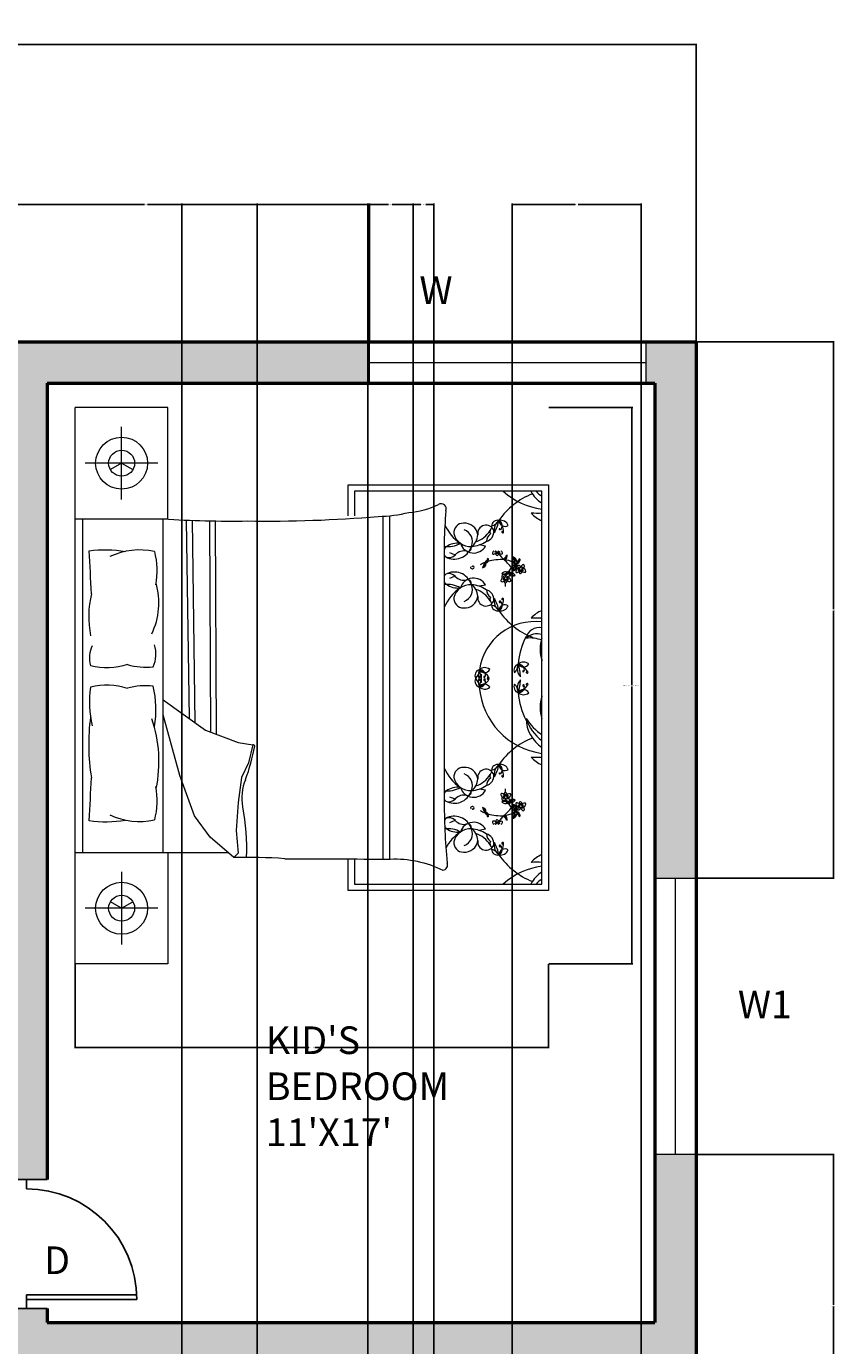
# Model space of a CAD drawing. Units: inches. Extents: x -55 to 413, y -498 to 86.
# Tile 6 of 6: x 238 to 413, y -201 to 86. Entities that reach past the tile are written whole.
import ezdxf

# ---------------------------------------------------------------- set-up
doc = ezdxf.new("R2010")
doc.units = ezdxf.units.IN
doc.header["$MEASUREMENT"] = 0
for name, color, linetype, lineweight in [('A-ANNO-DIMS', 2, 'Continuous', 18), ('A-ANNO-TEXT', 7, 'Continuous', 25), ('A-AREA-IDEN', 7, 'Continuous', 25), ('A-DOOR', 3, 'Continuous', 25), ('A-FURN', 9, 'Continuous', 18), ('A-GLAZ', 4, 'Continuous', 18), ('A-WALL', 7, 'Continuous', 50), ('A-WALL-PATT', 8, 'Continuous', 13)]:
    doc.layers.add(name, color=color, linetype=linetype, lineweight=lineweight)
doc.styles.get("Standard").update_dxf_attribs({"font": 'arial.ttf'})
doc.dimstyles.get("Standard").update_dxf_attribs({"dimtxt": 0.18, "dimasz": 0.18, "dimexe": 0.18, "dimexo": 0.0625, "dimgap": 0.09, "dimtad": 0, "dimtih": 1, "dimtoh": 1, "dimdec": 0, "dimzin": 0, "dimdsep": 46, "dimlunit": 3, "dimtxsty": 'Standard', "dimcen": 0.09, "dimadec": 0, "dimazin": 0, "dimtfac": 1, "dimtdec": 0, "dimtofl": 0, "dimtmove": 0, "dimatfit": 3, "dimfxl": 1, "dimtolj": 1, "dimtzin": 0, "dimarcsym": 0})

# ---------------------------------------------------------------- blocks, each defined once
blk = doc.blocks.new('*D2')
at = {"layer": 'A-ANNO-DIMS', "color": 0, "lineweight": -2, "transparency": 16777216}
for p, q in [((23, 17.6), (23, 82.27)), ((23.18, 82.09), (197.82, 82.09)), ((382.82, 82.09), (208.18, 82.09)), ((383, 17.6), (383, 82.27))]:
    blk.add_line(p, q, dxfattribs=at)
at = {"layer": 'A-ANNO-DIMS', "color": 0, "transparency": 16777216}
for points in [[(23.18, 82.12), (23.18, 82.06), (23, 82.09)], [(382.82, 82.12), (382.82, 82.06), (383, 82.09)]]:
    blk.add_solid(points, dxfattribs=at)
at = {"layer": 'Defpoints', "color": 0, "transparency": 16777216}
for p in [(383, 82.09), (23, 17.54), (383, 17.54)]:
    blk.add_point(p, dxfattribs=at)
at = {"layer": 'A-ANNO-DIMS', "color": 0, "transparency": 16777216, "insert": (203, 82.09), "char_height": 6, "attachment_point": 5}
blk.add_mtext("\\A1;30'", dxfattribs=at)
blk = doc.blocks.new('BED-DOUBLE-WITH-NIGHTSTANDS')
for p, q in [((0, 0), (0, 120.84)), ((10.07, 100.86), (10.07, 116.65)), ((17.96, 108.75), (2.18, 108.75)), ((59.24, 97.34), (59.24, 104.05)), ((59.24, 104.05), (102.77, 104.05)), ((102.77, 104.05), (102.77, 15.95)), ((60.64, 102.65), (60.64, 97.32)), ((101.37, 102.65), (60.64, 102.65)), ((101.37, 17.35), (101.37, 102.65)), ((1.55, 96.67), (1.55, 24.17)), ((19.1, 24.17), (19.1, 96.67)), ((24.12, 96.35), (24.72, 53.32)), ((25.36, 96.3), (25.98, 52.42)), ((29.16, 96.24), (29.34, 50.35)), ((30.4, 96.24), (30.59, 49.88)), ((66.77, 97.22), (66.77, 22.78)), ((68.28, 97.33), (68.28, 22.78)), ((89.11, 90.74), (87.75, 91)), ((80.15, 84.95), (80.15, 35.89)), ((89.11, 82.29), (87.75, 82.03)), ((19.1, 57.36), (28.31, 50.74)), ((22.69, 40.95), (19.1, 54.13)), ((28.31, 50.74), (35.41, 48.05)), ((35.41, 48.05), (38.59, 47.56)), ((38.59, 47.56), (37.61, 43.64)), ((37.61, 43.64), (36.14, 40.46)), ((25.87, 32.14), (22.69, 40.95)), ((36.14, 40.46), (35.41, 35.08)), ((89.11, 37.7), (87.75, 37.97)), ((35.41, 35.08), (34.92, 28.96)), ((29.29, 27.49), (25.87, 32.14)), ((34.92, 28.96), (35.41, 24.06)), ((89.11, 29.26), (87.75, 28.99)), ((34.43, 23.09), (29.29, 27.49)), ((0, 24.17), (33.17, 24.17)), ((35.41, 24.06), (34.43, 23.09)), ((59.24, 15.95), (59.24, 22.78)), ((60.64, 22.78), (60.64, 17.35)), ((10.07, 19.98), (10.07, 4.19)), ((60.64, 17.35), (101.37, 17.35)), ((102.77, 15.95), (59.24, 15.95)), ((17.96, 12.08), (2.18, 12.08))]:
    blk.add_line(p, q)
for points in [[(0, 96.67), (20.14, 96.67), (20.14, 120.84), (0, 120.84)], [(10.07, 108.75), (7.63, 107.35)], [(10.07, 108.75), (12.51, 107.35)], [(20.14, 24.17), (20.14, 0), (0, 0)], [(10.07, 12.08), (7.63, 13.49)], [(10.07, 12.08), (12.51, 13.49)]]:
    blk.add_lwpolyline(points)
for points in [[(65.82, 97.19, 0.056112), (72.47, 98.06, 0.095341), (78.87, 99.76)], [(3.01, 89.73, -0.074897), (10.9, 89.58, 0.472817)], [(11.35, 65.01, -0.14099), (3.29, 64.77, -0.235245)], [(11.35, 59.85, 0.14099), (3.29, 60.09, 0.235245)], [(3.01, 31.11, 0.074897), (10.9, 31.25, -0.472817)], [(45.49, 22.83, 0.001242), (68.42, 22.78, -0.127202), (79.85, 20.35)]]:
    blk.add_lwpolyline(points, format="xyb")
for centre, radius in [((10.07, 108.75), 5.64), ((10.07, 108.75), 2.82), ((96.74, 85.77), 0.308), ((93.49, 83.76), 0.308), ((93.49, 36.24), 0.308), ((96.74, 34.23), 0.308), ((10.07, 12.08), 5.64), ((10.07, 12.08), 2.82)]:
    blk.add_circle(centre, radius)
for centre, radius, start, end in [((105.05, 87.4), 15.78, 111.4092, 145.6135), ((103.49, 114.39), 15.78, 228.1144, 262.255), ((105.6, 106.48), 7.69, 209.8884, 236.5383), ((107.04, 109.24), 9.58, 223.5186, 233.6964), ((79.49, 98.85), 1.1, 336.5219, 123.8264), ((197.68, 88.65), 117.59, 175.2402, 181.8035), ((103.83, 102.17), 6.42, 221.0454, 247.4453), ((100.38, 119.75), 21.83, 266.3481, 272.5919), ((33.86, 313.3), 217.13, 266.1, 270.9282), ((41.76, 379.4), 283.23, 269.1145, 274.8735), ((88.66, 99), 9.15, 203.6453, 236.3329), ((84.27, 93.67), 2.04, 88.9462, 185.5144), ((84.56, 92.84), 2.89, 7.1143, 95.0551), ((89.21, 93.5), 1.81, 19.1312, 189.736), ((91.18, 93.88), 1.11, 126.7319, 206.0245), ((91.72, 95.04), 1.31, 76.272, 177.0484), ((89.73, 97.71), 2.7, 284.7031, 328.6173), ((93.49, 94.28), 2.49, 125.7657, 194.5347), ((81.25, 98.7), 11.04, 332.8176, 347.4827), ((92.4, 94.6), 1.75, 20.9613, 102.2885), ((93.35, 96.35), 1.32, 181.7131, 301.5367), ((89.03, 93.68), 3.99, 2.0648, 41.1598), ((91.43, 95.17), 1.29, 316.2238, 62.3173), ((85.78, 94.3), 3.63, 193.079, 274.7067), ((83.46, 91.7), 2.8, 338.5779, 68.4181), ((83.92, 93.34), 3.51, 305.9599, 357.6409), ((85.68, 97.15), 6.48, 273.4924, 303.7117), ((85.22, 97.1), 5.7, 288.2955, 328.7386), ((88.67, 93.94), 2.26, 285.6955, 4.031), ((91.68, 91.5), 2.41, 128.4175, 173.8338), ((92.17, 94.41), 0.103, 20.2667, 316.2271), ((92.82, 93.82), 0.196, 168.5166, 2.0648), ((92.72, 93.84), 0.0952, 52.0591, 168.5166), ((-1146.98, 23.12), 1151.92, 2.85022, 3.31479), ((14.07, 74.34), 15.57, 78.2417, 114.8684), ((1.6, 85.42), 16.19, 348.9631, 14.8961), ((81.49, 89.45), 1.46, 196.6343, 225.5483), ((81.49, 89.45), 1.46, 127.675, 162.5814), ((81.04, 95.65), 5.01, 259.249, 301.1782), ((82.34, 91.77), 3.85, 240.8249, 340.7178), ((81.2, 90.06), 1.81, 246.1646, 318.4347), ((83.22, 86.74), 4.66, 85.2696, 124.215), ((83.04, 92.35), 3.47, 240.0851, 262.564), ((84.4, 87.22), 2.48, 74.8529, 138.4347), ((86.51, 92.24), 3, 196.8663, 330.0915), ((85.25, 90.33), 0.75, 254.8529, 12.6959), ((83.22, 86.74), 4.66, 53.6555, 57.2989), ((90.82, 89.21), 0.238, 125.0752, 284.7644), ((91.19, 89.3), 0.513, 127.3642, 168.4363), ((90.79, 89.71), 0.74, 277.4968, 341.2737), ((91.37, 89.36), 0.294, 88.1325, 178.8919), ((91.96, 89.05), 0.636, 136.3462, 189.6513), ((91.6, 88.99), 0.265, 189.6513, 312.3208), ((91.66, 89.72), 0.308, 183.2768, 356.7232), ((92.63, 89.17), 1.01, 164.2829, 186.9148), ((91.44, 89.17), 0.504, 312.3208, 40.2111), ((92.5, 89.73), 0.715, 201.6382, 274.947), ((91.56, 88.75), 0.934, 42.3896, 66.5724), ((100.98, 96.15), 11.47, 217.9541, 226.8459), ((92.23, 89.3), 0.508, 10.9597, 52.2379), ((92.55, 89.26), 0.236, 274.947, 37.5263), ((86.24, 86.19), 0.379, 169.5864, 349.5616), ((86.38, 86.17), 0.233, 349.5616, 167.2949), ((92.47, 77.79), 10.01, 110.1059, 116.9968), ((89.11, 86.04), 0.634, 129.5056, 182.6421), ((87.29, 87.51), 1.91, 308.4388, 328.836), ((86.96, 89.06), 3.41, 296.5064, 305.3102), ((86.93, 87.31), 1.94, 336.3901, 344.4871), ((89.04, 86.81), 0.246, 83.9457, 185.6216), ((88.06, 87.04), 1.01, 328.836, 0.8141), ((88.58, 86.75), 0.58, 306.5232, 32.4668), ((89.27, 87.2), 0.246, 112.5583, 214.2343), ((89.11, 87.64), 0.58, 265.7131, 351.6568), ((88.6, 87.96), 1.01, 297.3659, 329.344), ((87.84, 88.83), 1.94, 313.6929, 321.7899), ((89.98, 87.5), 0.634, 115.5379, 168.6744), ((87.83, 88.42), 1.91, 329.344, 349.7412), ((92.47, 77.79), 10.01, 86.1723, 106.4158), ((86.31, 87.98), 3.41, 352.8698, 1.6736), ((93.34, 87.92), 0.246, 112.5583, 214.2343), ((93.18, 88.36), 0.58, 265.7131, 351.6568), ((92.67, 88.68), 1.01, 297.3659, 329.344), ((92.72, 82.78), 5.02, 60.7959, 85.244), ((82.04, 75.56), 16.51, 37.8256, 47.7588), ((91.9, 89.55), 1.94, 313.6929, 321.7899), ((94.05, 88.22), 0.634, 115.5379, 168.6744), ((91.9, 89.14), 1.91, 329.344, 349.7412), ((90.37, 88.7), 3.41, 352.8698, 1.6736), ((99.38, 82.26), 6.02, 130.182, 149.456), ((95.16, 88.01), 0.344, 33.0979, 123.1364), ((87.59, 83.16), 8.99, 31.1156, 34.8118), ((94.67, 87.42), 0.93, 2.3172, 70.5201), ((96.07, 85.69), 0.992, 139.3812, 199.9959), ((94.22, 86.41), 1.4, 310.9365, 22.7695), ((95.43, 87.19), 0.268, 135.7354, 318.1297), ((94.99, 87.63), 0.356, 315.7354, 31.1156), ((94.69, 86.87), 0.826, 319.3812, 5.5456), ((95.64, 87.19), 0.268, 68.2452, 250.6395), ((95.02, 87.52), 0.801, 352.6008, 57.1845), ((97.88, 82.14), 5.36, 111.7087, 116.2181), ((92.72, 82.78), 5.02, 47.5083, 55.9967), ((95.78, 87.7), 0.801, 252.8042, 349.6943), ((95.02, 86.27), 0.853, 331.1838, 51.6792), ((95.87, 87.77), 0.356, 248.2452, 323.6254), ((96.19, 86.16), 0.302, 138.2946, 276.2474), ((95.55, 87.99), 0.93, 291.7087, 3.0299), ((96.31, 86.11), 0.42, 358.5719, 143.8954), ((88.91, 92.89), 8.99, 323.6254, 327.3216), ((96.55, 86.44), 0.424, 208.8493, 269.9355), ((96.19, 86.34), 0.484, 274.2123, 318.1587), ((96.29, 87.75), 0.344, 325.6077, 55.6462), ((97.67, 85.85), 0.97, 121.9501, 165.2442), ((97, 86.23), 0.204, 262.868, 7.094), ((96.97, 86.4), 0.607, 278.5614, 22.5914), ((97.31, 86.42), 0.305, 44.3732, 121.9501), ((81.49, 83.58), 1.46, 134.4517, 156.7144), ((82.34, 81.26), 3.85, 19.2822, 119.1751), ((81.2, 82.97), 1.81, 41.5653, 113.8354), ((83.04, 80.68), 3.47, 97.436, 119.9149), ((84.4, 85.81), 2.48, 221.5653, 285.1471), ((86.51, 80.79), 3, 29.9085, 163.1337), ((85.25, 82.7), 0.75, 347.3041, 105.1471), ((92.65, 83.24), 0.238, 125.0752, 284.7644), ((93.02, 83.33), 0.513, 93.635, 168.4363), ((93.04, 86.11), 1.4, 253.6301, 325.4631), ((93.43, 84.17), 0.992, 82.0748, 142.6895), ((93.32, 85.53), 1.02, 228.342, 274.9894), ((92.95, 84.14), 0.302, 138.2946, 276.2474), ((92.61, 83.74), 0.74, 277.4968, 341.2737), ((93.06, 84.1), 0.42, 358.5719, 143.8954), ((93.2, 83.4), 0.294, 88.1325, 178.8919), ((93.31, 84.43), 0.424, 208.8493, 269.9355), ((92.95, 84.33), 0.484, 274.2123, 318.1587), ((93.79, 83.09), 0.636, 136.3462, 189.6513), ((93.35, 85.36), 0.853, 273.8774, 357.1501), ((94.45, 83.21), 1.01, 164.2829, 186.9148), ((94.42, 83.84), 0.97, 121.9501, 165.2442), ((93.68, 85.97), 0.826, 262.0748, 308.2393), ((93.27, 83.2), 0.504, 312.3208, 40.2111), ((94.33, 83.77), 0.715, 201.6382, 274.947), ((93.75, 84.21), 0.204, 262.868, 7.094), ((93.39, 82.79), 0.934, 42.3896, 66.5724), ((93.73, 84.38), 0.607, 278.5614, 22.5914), ((94.06, 83.34), 0.508, 10.9597, 118.7804), ((99.38, 82.26), 6.02, 156.1523, 156.9499), ((94.07, 84.4), 0.305, 44.3732, 121.9501), ((95.01, 85.12), 0.853, 181.4625, 249.4747), ((94.87, 85.79), 0.826, 215.1128, 261.2773), ((95.53, 85.75), 1.4, 197.889, 269.722), ((94.37, 83.29), 0.236, 274.947, 37.5263), ((95.09, 85.27), 1.02, 248.3627, 295.0101), ((94.59, 84), 0.992, 20.6625, 81.2773), ((94.86, 86.33), 1.02, 285.6484, 332.2957), ((95.89, 85.25), 0.238, 125.0752, 284.7644), ((96.26, 85.34), 0.513, 93.635, 168.4363), ((95.86, 85.76), 0.74, 277.4968, 341.2737), ((96.45, 85.41), 0.294, 88.1325, 178.8919), ((97.04, 85.1), 0.636, 136.3462, 189.6513), ((96.67, 85.04), 0.265, 189.6513, 312.3208), ((97.7, 85.22), 1.01, 164.2829, 186.9148), ((96.51, 85.21), 0.504, 312.3208, 40.2111), ((97.58, 85.78), 0.715, 201.6382, 274.947), ((96.63, 84.8), 0.934, 42.3896, 66.5724), ((97.31, 85.35), 0.508, 10.9597, 118.7804), ((97.62, 85.3), 0.236, 274.947, 37.5263), ((24.16, 75.39), 21.24, 166.3427, 191.1841), ((2.79, 78.43), 15.38, 333.8761, 16.1746), ((81.49, 83.58), 1.46, 203.2856, 232.325), ((81.04, 77.38), 5.01, 58.8218, 100.2867), ((88.66, 74.03), 9.15, 123.6671, 158.5059), ((83.22, 86.29), 4.66, 235.785, 274.7304), ((85.78, 78.73), 3.63, 85.2933, 166.921), ((83.46, 81.33), 2.8, 291.5819, 21.4221), ((83.22, 86.29), 4.66, 302.7011, 306.3445), ((83.92, 79.69), 3.51, 2.3591, 54.0401), ((85.68, 75.88), 6.48, 56.2883, 86.5076), ((85.22, 75.93), 5.7, 31.2614, 71.7045), ((91.68, 81.53), 2.41, 186.1662, 231.5825), ((88.67, 79.09), 2.26, 355.969, 74.3045), ((93.43, 83.02), 0.265, 189.6513, 312.3208), ((99.38, 82.26), 6.02, 175.2415, 182.8929), ((84.27, 79.36), 2.04, 174.4856, 271.0538), ((84.56, 80.19), 2.89, 264.9449, 352.8857), ((89.21, 79.53), 1.81, 170.264, 340.8688), ((91.18, 79.16), 1.11, 153.9755, 233.2681), ((91.72, 77.99), 1.31, 182.9516, 283.728), ((89.73, 75.32), 2.7, 31.3827, 75.2969), ((93.49, 78.75), 2.49, 165.4653, 234.2343), ((81.25, 74.33), 11.04, 12.5173, 27.1824), ((89.03, 79.35), 3.99, 318.8402, 357.9352), ((91.43, 77.86), 1.29, 297.6827, 43.7762), ((93.35, 76.68), 1.32, 58.4633, 178.2869), ((92.4, 78.43), 1.75, 257.7115, 339.0387), ((92.24, 78.64), 0.171, 43.7762, 339.7183), ((92.82, 79.21), 0.196, 357.9352, 191.4834), ((92.72, 79.19), 0.0952, 191.4834, 307.9409), ((105.05, 85.63), 15.78, 214.3865, 248.5908), ((103.83, 70.86), 6.42, 112.5547, 138.9546), ((100.38, 53.28), 21.83, 87.4081, 93.6519), ((99.85, 62.15), 12.21, 82.8636, 171.8197), ((100.7, 70.21), 2.83, 76.3898, 169.0739), ((100.31, 68.09), 3.58, 72.8609, 131.9049), ((9.04, 66.43), 5.98, 153.3437, 196.1026), ((11.12, 67.24), 6.41, 335.0183, 18.5407), ((111.94, 63.87), 15.78, 152.5854, 175.5377), ((98.73, 63.73), 7.06, 68.117, 96.6195), ((109.66, 68.29), 8.68, 162.9798, 196.4569), ((114.13, 64.85), 12.83, 174.3643, 175.6213), ((15.38, 79.26), 14.81, 254.1707, 275.9871), ((88.12, 62.64), 1.31, 106.1963, 206.9726), ((85.07, 63.96), 2.7, 314.6273, 358.5415), ((90.03, 62.87), 2.49, 155.6899, 224.4589), ((88.94, 62.6), 1.75, 50.8855, 132.2127), ((88.88, 64.58), 1.32, 211.6373, 331.4609), ((87.81, 62.6), 1.29, 346.148, 92.2415), ((86.47, 60.12), 3.99, 31.989, 71.0841), ((77.23, 60.59), 11.04, 2.7418, 17.407), ((96.58, 63.84), 1.31, 106.1963, 206.9726), ((93.52, 65.17), 2.7, 314.6273, 358.5415), ((98.49, 64.07), 2.49, 155.6899, 224.4589), ((97.39, 63.8), 1.75, 50.8855, 132.2127), ((97.33, 65.79), 1.32, 211.6373, 331.4609), ((94.92, 61.33), 3.99, 31.989, 71.0841), ((85.68, 61.8), 11.04, 2.7418, 17.407), ((96.26, 63.81), 1.29, 346.148, 92.2415), ((97.28, 63.53), 0.103, 50.1909, 346.0209), ((98.14, 63.34), 0.196, 198.4408, 31.989), ((98.04, 63.3), 0.0952, 81.9833, 198.4408), ((122.92, 58.09), 22.93, 160.0972, 160.2783), ((15.38, 45.61), 14.81, 84.0129, 105.8293), ((-3.78, 55.31), 21.31, 349.8617, 13.6238), ((88.12, 61.39), 1.31, 153.0274, 253.8037), ((85.07, 60.06), 2.7, 1.4585, 45.3727), ((90.03, 61.16), 2.49, 135.5411, 204.3101), ((77.23, 63.43), 11.04, 342.593, 357.2582), ((86.47, 63.91), 3.99, 288.9159, 328.011), ((87.81, 61.42), 1.29, 267.7585, 13.852), ((88.88, 59.44), 1.32, 28.5391, 148.3627), ((88.83, 62.32), 0.103, 50.1909, 346.0209), ((88.9, 61.69), 0.171, 13.852, 309.9245), ((89.59, 62.1), 0.0952, 81.9833, 198.4408), ((89.59, 61.93), 0.0952, 161.5592, 278.0167), ((89.68, 62.13), 0.196, 198.4408, 31.989), ((89.68, 61.9), 0.196, 328.011, 161.5592), ((96.58, 60.18), 1.31, 153.0274, 253.8037), ((93.52, 58.85), 2.7, 1.4585, 45.3727), ((98.49, 59.95), 2.49, 135.5411, 204.3101), ((85.68, 62.23), 11.04, 342.593, 357.2582), ((94.92, 62.7), 3.99, 288.9159, 328.011), ((96.26, 60.21), 1.29, 267.7585, 13.852), ((97.35, 60.48), 0.171, 13.852, 309.9245), ((98.14, 60.69), 0.196, 328.011, 161.5592), ((98.04, 60.72), 0.0952, 161.5592, 278.0167), ((24.59, 56.92), 21.53, 171.5249, 193.96), ((88.94, 61.43), 1.75, 227.7873, 309.1145), ((103.49, 61.36), 15.78, 184.4623, 262.255), ((97.33, 58.23), 1.32, 28.5391, 148.3627), ((97.39, 60.22), 1.75, 227.7873, 309.1145), ((111.94, 60.15), 15.78, 184.4623, 207.4146), ((109.66, 55.74), 8.68, 163.5431, 197.0202), ((114.13, 59.18), 12.83, 184.3787, 185.6357), ((122.92, 65.93), 22.93, 199.7217, 199.9028), ((46.74, 47.67), 43.83, 172.2196, 189.497), ((-9.91, 43.94), 28.09, 348.0397, 19.2615), ((105.6, 53.44), 7.69, 181.272, 236.5383), ((109.73, 61.24), 14.25, 214.0123, 234.053), ((107.04, 56.21), 9.58, 197.8504, 233.6964), ((105.05, 34.36), 15.78, 111.4092, 145.6135), ((-7.08, 55.95), 46.86, 340.1194, 349.3383), ((38.69, 47.29), 0.292, 358.8623, 109.7536), ((91.72, 42), 1.31, 76.272, 177.0484), ((89.73, 44.68), 2.7, 284.7031, 328.6173), ((93.49, 41.25), 2.49, 125.7657, 194.5347), ((81.25, 45.67), 11.04, 332.8176, 347.4827), ((92.4, 41.56), 1.75, 20.9613, 102.2885), ((91.43, 42.13), 1.29, 316.2238, 62.3173), ((89.03, 40.65), 3.99, 2.0648, 41.1598), ((93.35, 43.31), 1.32, 181.7131, 301.5367), ((100.38, 66.71), 21.83, 266.3481, 272.5919), ((103.83, 49.14), 6.42, 221.0454, 247.4453), ((-1146.98, 97.71), 1151.92, 356.68521, 357.14978), ((88.66, 45.97), 9.15, 201.4941, 236.3329), ((84.27, 40.64), 2.04, 88.9462, 185.5144), ((85.78, 41.27), 3.63, 193.079, 274.7067), ((84.56, 39.8), 2.89, 7.1143, 95.0551), ((83.46, 38.67), 2.8, 338.5779, 68.4181), ((83.92, 40.3), 3.51, 305.9599, 357.6409), ((85.22, 44.06), 5.7, 288.2955, 328.7386), ((89.21, 40.47), 1.81, 19.1312, 189.736), ((88.67, 40.9), 2.26, 285.6955, 4.031), ((91.68, 38.46), 2.41, 128.4175, 173.8338), ((91.18, 40.84), 1.11, 126.7319, 206.0245), ((92.17, 41.37), 0.103, 20.2667, 316.2271), ((92.82, 40.78), 0.196, 168.5166, 2.0648), ((92.72, 40.8), 0.0952, 52.0591, 168.5166), ((1.6, 35.42), 16.19, 345.1039, 11.0369), ((46, 36.05), 9.84, 156.2616, 191.3392), ((81.04, 42.61), 5.01, 259.7133, 301.1782), ((81.49, 36.41), 1.46, 127.675, 156.7144), ((82.34, 38.74), 3.85, 240.8249, 340.7178), ((83.22, 33.71), 4.66, 85.2696, 124.215), ((86.51, 39.2), 3, 196.8663, 330.0915), ((85.25, 37.3), 0.75, 254.8529, 12.6959), ((83.22, 33.71), 4.66, 53.6555, 57.2989), ((85.68, 44.12), 6.48, 273.4924, 303.7117), ((99.38, 37.73), 6.02, 177.1071, 184.7585), ((205.94, 34.45), 125.79, 179.3433, 185.6887), ((81.49, 36.41), 1.46, 203.229, 225.5483), ((81.2, 37.03), 1.81, 246.1646, 318.4347), ((83.04, 39.32), 3.47, 240.0851, 262.564), ((84.4, 34.18), 2.48, 74.8529, 138.4347), ((92.65, 36.76), 0.238, 75.2356, 234.9248), ((93.02, 36.66), 0.513, 191.5637, 266.365), ((93.32, 34.47), 1.02, 85.0106, 131.658), ((93.04, 33.88), 1.4, 34.5369, 106.3699), ((93.43, 35.83), 0.992, 217.3105, 277.9252), ((92.95, 35.85), 0.302, 83.7526, 221.7054), ((92.61, 36.25), 0.74, 18.7263, 82.5032), ((93.06, 35.9), 0.42, 216.1046, 1.4281), ((93.2, 36.6), 0.294, 181.1081, 271.8675), ((93.31, 35.57), 0.424, 90.0645, 151.1507), ((92.95, 35.67), 0.484, 41.8413, 85.7877), ((93.79, 36.91), 0.636, 170.3487, 223.6538), ((93.43, 36.97), 0.265, 47.6792, 170.3487), ((93.35, 34.63), 0.853, 2.8499, 86.1226), ((94.45, 36.79), 1.01, 173.0852, 195.7171), ((94.42, 36.16), 0.97, 194.7558, 238.0499), ((93.68, 34.03), 0.826, 51.7607, 97.9252), ((93.27, 36.8), 0.504, 319.7889, 47.6792), ((94.33, 36.23), 0.715, 85.053, 158.3618), ((93.75, 35.78), 0.204, 352.906, 97.132), ((93.39, 37.21), 0.934, 293.4276, 317.6104), ((94.06, 36.66), 0.508, 241.2196, 349.0403), ((93.73, 35.61), 0.607, 337.4086, 81.4386), ((99.38, 37.73), 6.02, 203.0501, 203.8477), ((94.07, 35.59), 0.305, 238.0499, 315.6268), ((95.01, 34.88), 0.853, 110.5253, 178.5375), ((95.53, 34.25), 1.4, 90.278, 162.111), ((94.87, 34.2), 0.826, 98.7227, 144.8872), ((99.38, 37.73), 6.02, 210.544, 229.818), ((94.37, 36.71), 0.236, 322.4737, 85.053), ((95.09, 34.73), 1.02, 64.9899, 111.6373), ((94.59, 36), 0.992, 278.7227, 339.3375), ((96.07, 34.31), 0.992, 160.0041, 220.6188), ((94.22, 33.59), 1.4, 337.2305, 49.0635), ((94.86, 33.66), 1.02, 27.7043, 74.3516), ((95.89, 34.74), 0.238, 75.2356, 234.9248), ((96.26, 34.65), 0.513, 191.5637, 266.365), ((95.86, 34.24), 0.74, 18.7263, 82.5032), ((96.45, 34.58), 0.294, 181.1081, 271.8675), ((97.04, 34.9), 0.636, 170.3487, 223.6538), ((96.67, 34.96), 0.265, 47.6792, 170.3487), ((97.7, 34.78), 1.01, 173.0852, 195.7171), ((96.51, 34.78), 0.504, 319.7889, 47.6792), ((97.58, 34.22), 0.715, 85.053, 158.3618), ((96.63, 35.19), 0.934, 293.4276, 317.6104), ((97.31, 34.65), 0.508, 241.2196, 349.0403), ((97.62, 34.69), 0.236, 322.4737, 85.053), ((14.07, 46.5), 15.57, 245.1316, 281.7583), ((-8.36, 25.15), 45.61, 357.4519, 11.3392), ((81.49, 30.55), 1.46, 134.4517, 153.558), ((82.34, 28.23), 3.85, 19.2822, 119.1751), ((81.2, 29.93), 1.81, 41.5653, 113.8354), ((86.24, 33.8), 0.379, 10.4384, 190.4136), ((86.38, 33.83), 0.233, 192.7051, 10.4384), ((92.47, 42.2), 10.01, 243.0032, 249.8941), ((87.29, 32.49), 1.91, 31.164, 51.5612), ((89.11, 33.95), 0.634, 177.3579, 230.4944), ((86.96, 30.93), 3.41, 54.6898, 63.4936), ((86.93, 32.69), 1.94, 15.5129, 23.6099), ((89.04, 33.18), 0.246, 174.3784, 276.0543), ((88.06, 32.95), 1.01, 359.1859, 31.164), ((88.58, 33.25), 0.58, 327.5332, 53.4768), ((89.27, 32.8), 0.246, 145.7657, 247.4417), ((89.11, 32.36), 0.58, 8.3432, 94.2869), ((88.6, 32.04), 1.01, 30.656, 62.6341), ((87.84, 31.17), 1.94, 38.2101, 46.3071), ((89.98, 32.49), 0.634, 191.3256, 244.4621), ((87.83, 31.58), 1.91, 10.2588, 30.656), ((92.47, 42.2), 10.01, 253.5842, 273.8277), ((86.31, 32.02), 3.41, 358.3264, 7.1302), ((100.98, 23.85), 11.47, 133.1541, 142.0459), ((93.34, 32.08), 0.246, 145.7657, 247.4417), ((82.04, 44.44), 16.51, 312.2412, 322.1744), ((92.72, 37.22), 5.02, 274.756, 299.2041), ((93.18, 31.64), 0.58, 8.3432, 94.2869), ((92.67, 31.32), 1.01, 30.656, 62.6341), ((91.9, 30.45), 1.94, 38.2101, 46.3071), ((94.05, 31.77), 0.634, 191.3256, 244.4621), ((91.9, 30.86), 1.91, 10.2588, 30.656), ((90.37, 31.3), 3.41, 358.3264, 7.1302), ((94.67, 32.58), 0.93, 289.4799, 357.6828), ((87.59, 36.83), 8.99, 325.1882, 328.8844), ((95.16, 31.99), 0.344, 236.8636, 326.9021), ((95.43, 32.81), 0.268, 41.8703, 224.2646), ((94.99, 32.37), 0.356, 328.8844, 44.2646), ((94.69, 33.12), 0.826, 354.4544, 40.6188), ((95.64, 32.8), 0.268, 109.3605, 291.7548), ((95.02, 32.47), 0.801, 302.8155, 7.3992), ((97.88, 37.85), 5.36, 243.7819, 248.2913), ((92.72, 37.22), 5.02, 304.0033, 312.4917), ((95.02, 33.73), 0.853, 308.3208, 28.8162), ((95.78, 32.29), 0.801, 10.3057, 107.1958), ((95.87, 32.22), 0.356, 36.3746, 111.7548), ((96.19, 33.84), 0.302, 83.7526, 221.7054), ((95.55, 32.01), 0.93, 356.9701, 68.2913), ((96.31, 33.89), 0.42, 216.1046, 1.4281), ((88.91, 27.1), 8.99, 32.6784, 36.3746), ((96.55, 33.56), 0.424, 90.0645, 151.1507), ((96.19, 33.66), 0.484, 41.8413, 85.7877), ((96.29, 32.24), 0.344, 304.3538, 34.3923), ((97.67, 34.14), 0.97, 194.7558, 238.0499), ((97, 33.77), 0.204, 352.906, 97.132), ((96.97, 33.6), 0.607, 337.4086, 81.4386), ((97.31, 33.58), 0.305, 238.0499, 315.6268), ((81.49, 30.55), 1.46, 210.0293, 232.325), ((81.04, 24.35), 5.01, 58.8218, 99.1554), ((83.22, 33.25), 4.66, 235.785, 274.7304), ((83.04, 27.64), 3.47, 97.436, 119.9149), ((85.78, 25.7), 3.63, 85.2933, 166.921), ((84.4, 32.78), 2.48, 221.5653, 285.1471), ((86.51, 27.76), 3, 29.9085, 163.1337), ((83.46, 28.29), 2.8, 291.5819, 21.4221), ((85.25, 29.66), 0.75, 347.3041, 105.1471), ((83.22, 33.25), 4.66, 302.7011, 306.3445), ((83.92, 26.66), 3.51, 2.3591, 54.0401), ((85.68, 22.84), 6.48, 56.2883, 86.5076), ((90.82, 30.79), 0.238, 75.2356, 234.9248), ((91.19, 30.7), 0.513, 191.5637, 232.6358), ((90.79, 30.29), 0.74, 18.7263, 82.5032), ((91.37, 30.63), 0.294, 181.1081, 271.8675), ((91.96, 30.94), 0.636, 170.3487, 223.6538), ((91.6, 31.01), 0.265, 47.6792, 170.3487), ((91.66, 30.27), 0.308, 3.2768, 176.7232), ((92.63, 30.82), 1.01, 173.0852, 195.7171), ((91.44, 30.83), 0.504, 319.7889, 47.6792), ((92.5, 30.26), 0.715, 85.053, 158.3618), ((91.56, 31.24), 0.934, 293.4276, 317.6104), ((92.23, 30.69), 0.508, 307.7621, 349.0403), ((92.55, 30.74), 0.236, 322.4737, 85.053), ((88.66, 20.99), 9.15, 123.6671, 153.2997), ((84.27, 26.32), 2.04, 174.4856, 271.0538), ((84.56, 27.16), 2.89, 264.9449, 352.8857), ((85.22, 22.9), 5.7, 31.2614, 71.7045), ((89.21, 26.49), 1.81, 170.264, 340.8688), ((88.67, 26.06), 2.26, 355.969, 74.3045), ((91.68, 28.5), 2.41, 186.1662, 231.5825), ((91.18, 26.12), 1.11, 153.9755, 233.2681), ((93.49, 25.71), 2.49, 165.4653, 234.2343), ((81.25, 21.29), 11.04, 12.5173, 27.1824), ((89.03, 26.31), 3.99, 318.8402, 357.9352), ((92.82, 26.18), 0.196, 357.9352, 191.4834), ((92.72, 26.16), 0.0952, 191.4834, 307.9409), ((37.43, -87.71), 110.84, 85.8294, 91.553), ((89.73, 22.28), 2.7, 31.3827, 75.2969), ((91.72, 24.96), 1.31, 182.9516, 283.728), ((91.43, 24.83), 1.29, 297.6827, 43.7762), ((93.35, 23.65), 1.32, 58.4633, 178.2869), ((92.4, 25.4), 1.75, 257.7115, 339.0387), ((105.05, 32.6), 15.78, 214.3865, 248.5908), ((92.24, 25.6), 0.171, 43.7762, 339.7183), ((103.83, 17.82), 6.42, 112.5547, 138.9546), ((79.77, 21.46), 1.11, 273.98, 27.3412), ((103.49, 5.6), 15.78, 97.745, 131.8856), ((100.38, 0.25), 21.83, 87.4081, 93.6519), ((105.6, 13.52), 7.69, 123.4617, 150.1116), ((107.04, 10.75), 9.58, 126.3036, 136.4814)]:
    blk.add_arc(centre, radius, start, end)
blk = doc.blocks.new('DOOR-SINGLE-24')
for p, q in [((24, 28), (19.5, 28)), ((24, 26), (24, 28)), ((24, 28), (28.5, 28)), ((24, 3), (0, 3)), ((24, 3), (24, 2)), ((24, 2), (0, 2)), ((24, 0), (24, 2)), ((19.5, 0), (28.5, 0))]:
    blk.add_line(p, q)
blk.add_arc((24, 2), 24, 90, 180)
blk = doc.blocks.new('WIN-60IN')
for p, q in [((0, 9), (60, 9)), ((0, 0), (0, 9)), ((60, 9), (60, 0)), ((0, 4.5), (60, 4.5)), ((60, 0), (0, 0))]:
    blk.add_line(p, q)
blk = doc.blocks.new('*D19')
at = {"layer": 'A-ANNO-DIMS', "color": 0, "lineweight": -2, "transparency": 16777216}
for p, q in [((350.95, 3.24), (369.19, 3.24)), ((369.01, 3.06), (369.01, -57)), ((369.01, -117.42), (369.01, -57.36)), ((350.95, -117.6), (369.19, -117.6))]:
    blk.add_line(p, q, dxfattribs=at)
at = {"layer": 'A-ANNO-DIMS', "color": 0, "transparency": 16777216}
for points in [[(368.98, 3.06), (369.04, 3.06), (369.01, 3.24)], [(368.98, -117.42), (369.04, -117.42), (369.01, -117.6)]]:
    blk.add_solid(points, dxfattribs=at)
at = {"layer": 'Defpoints', "color": 0, "transparency": 16777216}
for p in [(350.88, 3.24), (369.01, 3.24), (350.88, -117.6)]:
    blk.add_point(p, dxfattribs=at)
at = {"layer": 'A-ANNO-DIMS', "color": 0, "transparency": 16777216, "insert": (369.01, -57.18), "char_height": 0.18, "attachment_point": 5}
blk.add_mtext('\\A1;BED & NIGHTSTANDS 10\'-1" TYP.', dxfattribs=at)
blk = doc.blocks.new('*D20')
at = {"layer": 'A-ANNO-DIMS', "color": 0, "lineweight": -2, "transparency": 16777216}
for p, q in [((248.12, -117.66), (248.12, -135.91)), ((350.88, -117.66), (350.88, -135.91)), ((248.3, -135.73), (298.86, -135.73)), ((350.7, -135.73), (300.14, -135.73))]:
    blk.add_line(p, q, dxfattribs=at)
at = {"layer": 'A-ANNO-DIMS', "color": 0, "transparency": 16777216}
for points in [[(248.3, -135.7), (248.3, -135.76), (248.12, -135.73)], [(350.7, -135.7), (350.7, -135.76), (350.88, -135.73)]]:
    blk.add_solid(points, dxfattribs=at)
at = {"layer": 'Defpoints', "color": 0, "transparency": 16777216}
for p in [(248.12, -117.6), (350.88, -117.6), (350.88, -135.73)]:
    blk.add_point(p, dxfattribs=at)
at = {"layer": 'A-ANNO-DIMS', "color": 0, "transparency": 16777216, "insert": (299.5, -135.73), "char_height": 0.18, "attachment_point": 5}
blk.add_mtext('\\A1;8\'-7" TYP.', dxfattribs=at)
blk = doc.blocks.new('*D29')
at = {"layer": 'A-ANNO-DIMS', "color": 0, "lineweight": -2, "transparency": 16777216}
for p, q in [((215, 17.6), (215, 47.52)), ((215.18, 47.34), (263.19, 47.34)), ((311.85, 47.34), (263.84, 47.34)), ((312.03, 17.6), (312.03, 47.52))]:
    blk.add_line(p, q, dxfattribs=at)
at = {"layer": 'A-ANNO-DIMS', "color": 0, "transparency": 16777216}
for points in [[(215.18, 47.37), (215.18, 47.31), (215, 47.34)], [(311.85, 47.37), (311.85, 47.31), (312.03, 47.34)]]:
    blk.add_solid(points, dxfattribs=at)
at = {"layer": 'Defpoints', "color": 0, "transparency": 16777216}
for p in [(312.03, 47.34), (215, 17.54), (312.03, 17.54)]:
    blk.add_point(p, dxfattribs=at)
at = {"layer": 'A-ANNO-DIMS', "color": 0, "transparency": 16777216, "insert": (263.52, 47.34), "char_height": 0.18, "attachment_point": 5}
blk.add_mtext('\\A1;8\'-1"', dxfattribs=at)
blk = doc.blocks.new('*D33')
at = {"layer": 'A-ANNO-DIMS', "color": 0, "lineweight": -2, "transparency": 16777216}
for p, q in [((383.07, 17.54), (412.98, 17.54)), ((412.8, 17.36), (412.8, -40.55)), ((412.8, -98.83), (412.8, -40.92)), ((383.07, -99.01), (412.98, -99.01))]:
    blk.add_line(p, q, dxfattribs=at)
at = {"layer": 'A-ANNO-DIMS', "color": 0, "transparency": 16777216}
for points in [[(412.77, 17.36), (412.83, 17.36), (412.8, 17.54)], [(412.77, -98.83), (412.83, -98.83), (412.8, -99.01)]]:
    blk.add_solid(points, dxfattribs=at)
at = {"layer": 'Defpoints', "color": 0, "transparency": 16777216}
for p in [(383, 17.54), (412.8, 17.54), (383, -99.01)]:
    blk.add_point(p, dxfattribs=at)
at = {"layer": 'A-ANNO-DIMS', "color": 0, "transparency": 16777216, "insert": (412.8, -40.74), "char_height": 0.18, "attachment_point": 5}
blk.add_mtext('\\A1;9\'-8 1/2"', dxfattribs=at)
blk = doc.blocks.new('*D34')
at = {"layer": 'A-ANNO-DIMS', "color": 0, "lineweight": -2, "transparency": 16777216}
for p, q in [((383.07, -159.01), (412.98, -159.01)), ((412.8, -159.19), (412.8, -191.68)), ((412.8, -224.53), (412.8, -192.04)), ((383.07, -224.71), (412.98, -224.71))]:
    blk.add_line(p, q, dxfattribs=at)
at = {"layer": 'A-ANNO-DIMS', "color": 0, "transparency": 16777216}
for points in [[(412.77, -159.19), (412.83, -159.19), (412.8, -159.01)], [(412.77, -224.53), (412.83, -224.53), (412.8, -224.71)]]:
    blk.add_solid(points, dxfattribs=at)
at = {"layer": 'Defpoints', "color": 0, "transparency": 16777216}
for p in [(383, -159.01), (383, -224.71), (412.8, -224.71)]:
    blk.add_point(p, dxfattribs=at)
at = {"layer": 'A-ANNO-DIMS', "color": 0, "transparency": 16777216, "insert": (412.8, -191.86), "char_height": 0.18, "attachment_point": 5}
blk.add_mtext('\\A1;5\'-5 1/2"', dxfattribs=at)
blk = doc.blocks.new('*D36')
at = {"layer": 'A-ANNO-DIMS', "color": 0, "lineweight": -2, "transparency": 16777216}
for p, q in [((343, -280.9), (343, 47.52)), ((343.18, 47.34), (356.67, 47.34)), ((370.82, 47.34), (357.33, 47.34)), ((371, -280.9), (371, 47.52))]:
    blk.add_line(p, q, dxfattribs=at)
at = {"layer": 'A-ANNO-DIMS', "color": 0, "transparency": 16777216}
for points in [[(343.18, 47.37), (343.18, 47.31), (343, 47.34)], [(370.82, 47.37), (370.82, 47.31), (371, 47.34)]]:
    blk.add_solid(points, dxfattribs=at)
at = {"layer": 'Defpoints', "color": 0, "transparency": 16777216}
for p in [(371, 47.34), (343, -280.96), (371, -280.96)]:
    blk.add_point(p, dxfattribs=at)
at = {"layer": 'A-ANNO-DIMS', "color": 0, "transparency": 16777216, "insert": (357, 47.34), "char_height": 0.18, "attachment_point": 5}
blk.add_mtext('\\A1;2\'-4"', dxfattribs=at)
blk = doc.blocks.new('*D37')
at = {"layer": 'A-ANNO-DIMS', "color": 0, "lineweight": -2, "transparency": 16777216}
for p, q in [((321.5, -280.9), (321.5, 47.52)), ((321.68, 47.34), (323.21, 47.34)), ((325.82, 47.34), (324.29, 47.34)), ((326, -285.4), (326, 47.52))]:
    blk.add_line(p, q, dxfattribs=at)
at = {"layer": 'A-ANNO-DIMS', "color": 0, "transparency": 16777216}
for points in [[(321.68, 47.37), (321.68, 47.31), (321.5, 47.34)], [(325.82, 47.37), (325.82, 47.31), (326, 47.34)]]:
    blk.add_solid(points, dxfattribs=at)
at = {"layer": 'Defpoints', "color": 0, "transparency": 16777216}
for p in [(326, 47.34), (321.5, -280.96), (326, -285.46)]:
    blk.add_point(p, dxfattribs=at)
at = {"layer": 'A-ANNO-DIMS', "color": 0, "transparency": 16777216, "insert": (323.75, 47.34), "char_height": 0.18, "attachment_point": 5}
blk.add_mtext('\\A1;0\'-4 1/2"', dxfattribs=at)
blk = doc.blocks.new('*D39')
at = {"layer": 'A-ANNO-DIMS', "color": 0, "lineweight": -2, "transparency": 16777216}
for p, q in [((271.25, -357.4), (271.25, 47.52)), ((271.43, 47.34), (278.91, 47.34)), ((287.45, 47.34), (279.97, 47.34)), ((287.63, -357.4), (287.63, 47.52))]:
    blk.add_line(p, q, dxfattribs=at)
at = {"layer": 'A-ANNO-DIMS', "color": 0, "transparency": 16777216}
for points in [[(271.43, 47.37), (271.43, 47.31), (271.25, 47.34)], [(287.45, 47.37), (287.45, 47.31), (287.63, 47.34)]]:
    blk.add_solid(points, dxfattribs=at)
at = {"layer": 'Defpoints', "color": 0, "transparency": 16777216}
for p in [(287.63, 47.34), (271.25, -357.46), (287.63, -357.46)]:
    blk.add_point(p, dxfattribs=at)
at = {"layer": 'A-ANNO-DIMS', "color": 0, "transparency": 16777216, "insert": (279.44, 47.34), "char_height": 0.18, "attachment_point": 5}
blk.add_mtext('\\A1;1\'-4 1/2"', dxfattribs=at)
blk = doc.blocks.new('*D42')
at = {"layer": 'A-ANNO-DIMS', "color": 0, "lineweight": -2, "transparency": 16777216}
for p, q in [((311.63, -357.4), (311.63, 47.52)), ((311.81, 47.34), (316.17, 47.34)), ((321.32, 47.34), (316.97, 47.34)), ((321.5, -357.4), (321.5, 47.52))]:
    blk.add_line(p, q, dxfattribs=at)
at = {"layer": 'A-ANNO-DIMS', "color": 0, "transparency": 16777216}
for points in [[(311.81, 47.37), (311.81, 47.31), (311.63, 47.34)], [(321.32, 47.37), (321.32, 47.31), (321.5, 47.34)]]:
    blk.add_solid(points, dxfattribs=at)
at = {"layer": 'Defpoints', "color": 0, "transparency": 16777216}
for p in [(321.5, 47.34), (311.63, -357.46), (321.5, -357.46)]:
    blk.add_point(p, dxfattribs=at)
at = {"layer": 'A-ANNO-DIMS', "color": 0, "transparency": 16777216, "insert": (316.57, 47.34), "char_height": 0.18, "attachment_point": 5}
blk.add_mtext('\\A1;0\'-10"', dxfattribs=at)

msp = doc.modelspace()

# ---------------------------------------------------------------- hatches: boundary and pattern name
at = {"layer": 'A-WALL-PATT'}
h = msp.add_hatch(color=256, dxfattribs=at)
h.dxf.hatch_style = 1
h.paths.add_polyline_path([(97.55, 17.54), (23, 17.54), (23, -94.08), (32, -94.08), (32, 8.54), (97.55, 8.54)])
h.paths.add_polyline_path([(191, 17.54), (157.55, 17.54), (157.55, 8.54), (164, 8.54), (164, -80.46), (168.5, -80.46), (173, -80.46), (173, 8.54), (191, 8.54)])
h.paths.add_polyline_path([(312.03, 17.54), (215, 17.54), (215, 8.54), (233, 8.54), (233, -111.46), (173, -111.46), (173, -108.46), (164, -108.46), (164, -164.46), (168.5, -164.46), (173, -164.46), (173, -120.46), (233, -120.46), (233, -164.46), (237.5, -164.46), (242, -164.46), (242, 8.54), (312.03, 8.54)])
h.paths.add_polyline_path([(383, 17.54), (372.03, 17.54), (372.03, 8.54), (374, 8.54), (374, -99.01), (383, -99.01)])
h.paths.add_polyline_path([(383, -159.01), (374, -159.01), (374, -195.46), (242, -195.46), (242, -192.46), (233, -192.46), (233, -204.46), (374, -204.46), (374, -224.71), (383, -224.71)])
h.paths.add_polyline_path([(173, -192.46), (164, -192.46), (164, -195.46), (32, -195.46), (32, -154.08), (23, -154.08), (23, -213.4), (32, -213.4), (32, -204.46), (164, -204.46), (164, -221.46), (168.5, -221.46), (173, -221.46)])
h.paths.add_polyline_path([(173, -249.46), (164, -249.46), (164, -252.46), (32, -252.46), (32, -237.4), (23, -237.4), (23, -273.22), (32, -273.22), (32, -261.46), (164, -261.46), (173, -261.46)])
h.paths.add_polyline_path([(32, -309.22), (23, -309.22), (23, -456.46), (23, -460.96), (199.52, -460.96), (199.52, -456.46), (32, -456.46), (32, -366.46), (97.71, -366.46), (97.71, -357.46), (32, -357.46)])
h.paths.add_polyline_path([(188.35, -357.46), (173, -357.46), (173, -302.07), (164, -302.07), (164, -357.46), (157.71, -357.46), (157.71, -366.46), (188.35, -366.46)])
h.paths.add_polyline_path([(223.25, -357.46), (212.35, -357.46), (212.35, -366.46), (223.25, -366.46), (223.25, -361.96)])
h.paths.add_polyline_path([(287.63, -357.46), (271.25, -357.46), (271.25, -361.96), (271.25, -366.46), (287.63, -366.46)])
h.paths.add_polyline_path([(374, -357.46), (311.63, -357.46), (311.63, -366.46), (374, -366.46)])
h.paths.add_polyline_path([(383, -456.46), (383, -366.46), (378.5, -366.46), (378.5, -456.46), (309.45, -456.46), (309.45, -460.96), (383, -460.96)])
h.paths.add_polyline_path([(309.45, -458.71), (199.52, -458.71), (199.52, -460.96), (309.45, -460.96)])
h.paths.add_polyline_path([(383, -260.71), (374, -260.71), (374, -280.96), (371, -280.96), (371, -285.46), (374, -285.46), (374, -366.46), (383, -366.46)])
h.paths.add_polyline_path([(343, -283.21), (343, -280.96), (321.5, -280.96), (321.5, -357.46), (326, -357.46), (326, -285.46), (343, -285.46)])

# ---------------------------------------------------------------- linework, layer by layer
at = {"layer": 'A-WALL'}
for p, q in [((23, 17.54), (383, 17.54)), ((383, 17.54), (383, -456.46)), ((242, 8.54), (242, -164.46)), ((242, 8.54), (374, 8.54)), ((374, 8.54), (374, -195.46)), ((242, -192.46), (242, -195.46)), ((242, -195.46), (374, -195.46))]:
    msp.add_line(p, q, dxfattribs=at)

# ---------------------------------------------------------------- block references
at = {"layer": 'A-DOOR', "extrusion": (0, 0, -1), "zscale": -1}
msp.add_blockref('DOOR-SINGLE-24', (-261.5, -192.46), dxfattribs=at)
at = {"layer": 'A-FURN'}
msp.add_blockref('BED-DOUBLE-WITH-NIGHTSTANDS', (248.12, -117.6), dxfattribs=at)
at = {"layer": 'A-GLAZ'}
msp.add_blockref('WIN-60IN', (312.03, 8.54), dxfattribs=at)
at = {"layer": 'A-GLAZ', "rotation": 90.00000000000003}
msp.add_blockref('WIN-60IN', (383, -159.01), dxfattribs=at)

# ---------------------------------------------------------------- texts
at = {"layer": 'A-ANNO-TEXT', "char_height": 6, "attachment_point": 1}
for s, insert in [('W', (322.87, 31.7)), ('W1', (392.04, -123.42)), ('D', (241.36, -178.97))]:
    msp.add_mtext(s, dxfattribs=dict(at, insert=insert))
at = {"layer": 'A-AREA-IDEN', "insert": (289.51, -131.18), "char_height": 6, "attachment_point": 1}
msp.add_mtext("KID'S\\PBEDROOM\\P11'X17'", dxfattribs=at)

# ---------------------------------------------------------------- dimensions: what is measured, and where the dimension line sits
at = {"layer": 'A-ANNO-DIMS'}
for base, p1, p2, override, picture, middle in [((383, 82.09), (23, 17.54), (383, 17.54), {"dimtxt": 6, "dimclrd": 0, "dimclre": 0, "dimclrt": 0}, '*D2', (203, 82.09)), ((312.03, 47.34), (215, 17.54), (312.03, 17.54), {"dimdec": 1, "dimlfac": 1, "dimrnd": 0, "dimzin": 1, "dimdsep": 46, "dimlunit": 4, "dimfrac": 2}, '*D29', (263.52, 47.34)), ((287.63, 47.34), (271.25, -357.46), (287.63, -357.46), {"dimdec": 1, "dimlfac": 1, "dimrnd": 0, "dimzin": 1, "dimdsep": 46, "dimlunit": 4, "dimfrac": 2}, '*D39', (279.44, 47.34)), ((321.5, 47.34), (311.63, -357.46), (321.5, -357.46), {"dimdec": 1, "dimlfac": 1, "dimrnd": 0, "dimzin": 1, "dimdsep": 46, "dimlunit": 4, "dimfrac": 2}, '*D42', (316.57, 47.34)), ((326, 47.34), (321.5, -280.96), (326, -285.46), {"dimdec": 1, "dimlfac": 1, "dimrnd": 0, "dimzin": 1, "dimdsep": 46, "dimlunit": 4, "dimfrac": 2}, '*D37', (323.75, 47.34)), ((371, 47.34), (343, -280.96), (371, -280.96), {"dimdec": 1, "dimlfac": 1, "dimrnd": 0, "dimzin": 1, "dimdsep": 46, "dimlunit": 4, "dimfrac": 2}, '*D36', (357, 47.34))]:
    dim = msp.add_linear_dim(base=base, p1=p1, p2=p2, dimstyle='Standard', override=override, dxfattribs=at)
    dim.commit()
    dim.dimension.update_dxf_attribs({"geometry": picture, "text_midpoint": middle})
for base, p1, p2, picture, middle in [((412.8027, 17.5397), (383.0027, -99.0101), (383.0027, 17.5397), '*D33', (412.8027, -40.7352)), ((412.8, -224.71), (383, -159.01), (383, -224.71), '*D34', (412.8, -191.86))]:
    dim = msp.add_linear_dim(base=base, p1=p1, p2=p2, angle=90, dimstyle='Standard', override={"dimdec": 1, "dimlfac": 1, "dimrnd": 0, "dimzin": 1, "dimdsep": 46, "dimlunit": 4, "dimfrac": 2}, dxfattribs=at)
    dim.commit()
    dim.dimension.update_dxf_attribs({"geometry": picture, "text_midpoint": middle})
dim = msp.add_linear_dim(base=(369.01, 3.24), p1=(350.88, -117.6), p2=(350.88, 3.24), angle=90, text='BED & NIGHTSTANDS <> TYP.', dimstyle='Standard', override={"dimdec": 1, "dimlfac": 1, "dimrnd": 0, "dimzin": 1, "dimdsep": 46, "dimlunit": 4, "dimfrac": 2}, dxfattribs=at)
dim.commit()
dim.dimension.update_dxf_attribs({"geometry": '*D19', "text_midpoint": (369.01, -57.18)})
dim = msp.add_linear_dim(base=(350.88, -135.73), p1=(248.12, -117.6), p2=(350.88, -117.6), text='<> TYP.', dimstyle='Standard', override={"dimdec": 1, "dimlfac": 1, "dimrnd": 0, "dimzin": 1, "dimdsep": 46, "dimlunit": 4, "dimfrac": 2}, dxfattribs=at)
dim.commit()
dim.dimension.update_dxf_attribs({"geometry": '*D20', "text_midpoint": (299.5, -135.73)})

doc.saveas('drawing.dxf')
